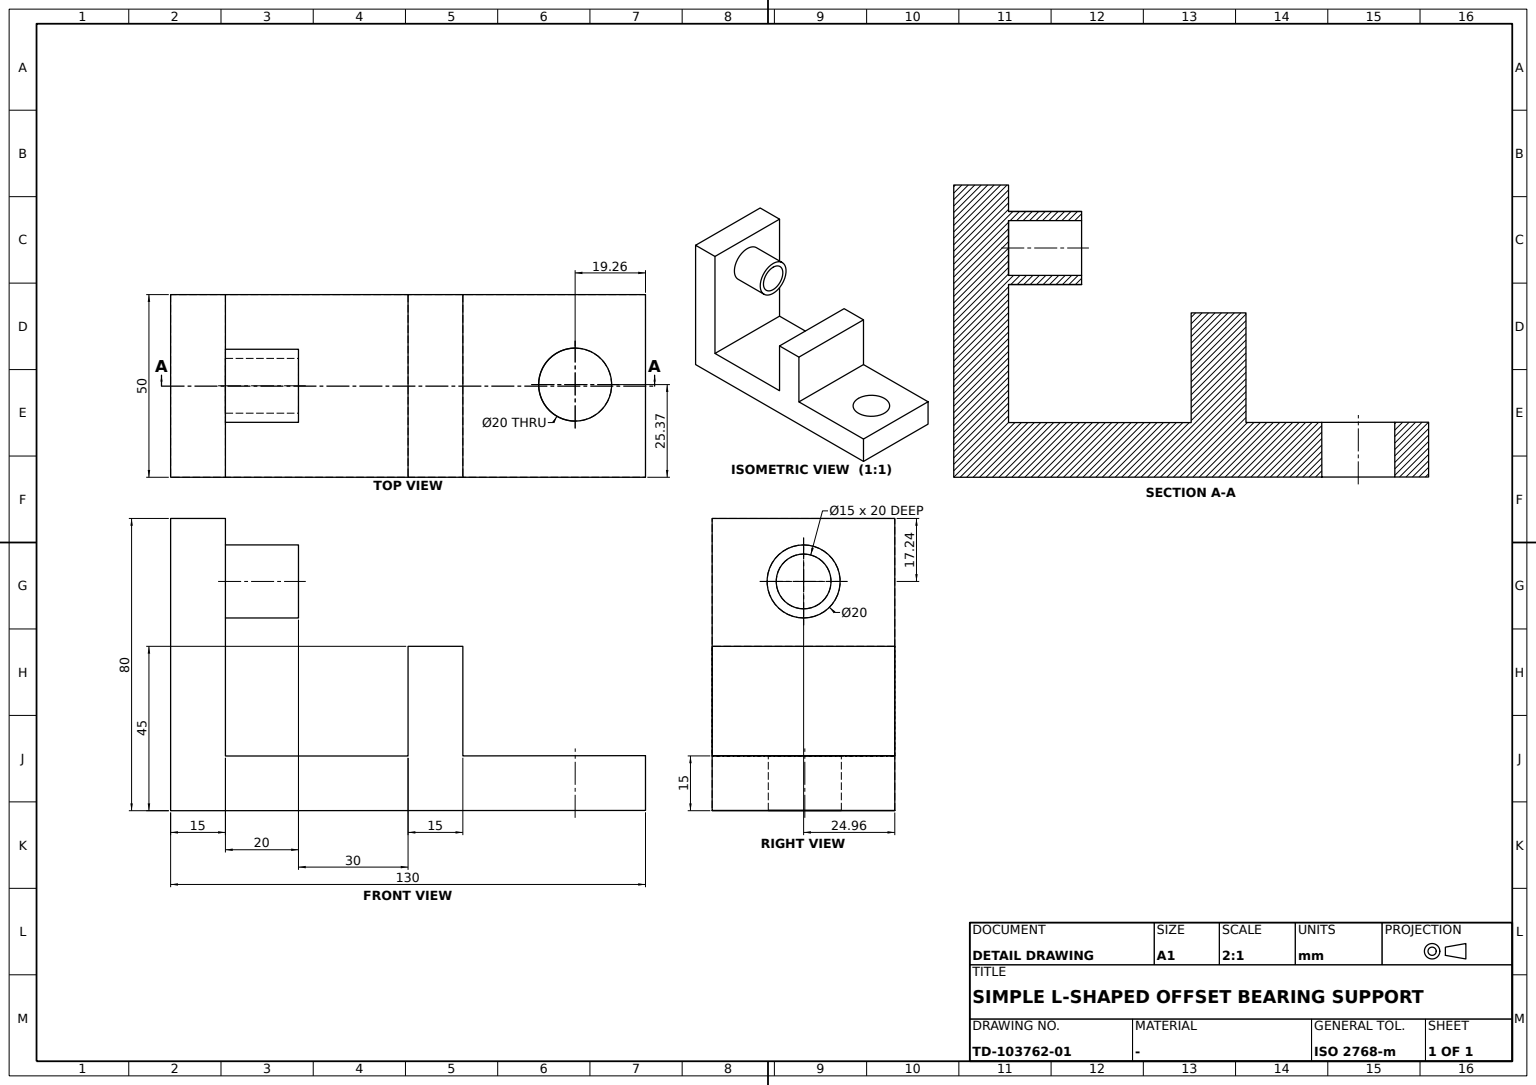
CATIA V5 part; units mm, degrees
sketch "Sketch1" plane through (0, 0, 0) normal (1, 0, 0) x (0, 1, 0)
  line L0 (0, 0) -> (130, 0.0732)
  line L1 (130, 0.0732) -> (130, 15.0732)
  line L2 (130, 15.0732) -> (80, 14.9978)
  line L3 (80, 14.9978) -> (80, 44.9978)
  line L4 (80, 44.9978) -> (65, 44.9978)
  line L5 (65, 44.9978) -> (65, 14.9751)
  line L6 (0, 0) -> (0, 80)
  line L7 (0, 80) -> (15, 80)
  line L8 (15, 80) -> (15, 14.9751)
  line L9 (65, 14.9751) -> (15, 14.9751)
  dimension "length L0" = 130
  dimension "length L1" = 15
  dimension "length L2" = 50
  dimension "length L3" = 30
  dimension "length L4" = 15
  dimension "length L6" = 80
  dimension "length L7" = 15
extrude "Pad1" add sketch "Sketch1" along normal blind 50
sketch "Sketch3" plane through (0, 15, 0) normal (0, 1, 0) x (-1, 0, 0)
  circle A0 centre (-24.9594, 62.7568) radius 10
  circle A1 centre (-24.9594, 62.7568) radius 7.5
  dimension "radius A0" = 10
  dimension "radius A1" = 7.5
extrude "Pad2" add sketch "Sketch3" along normal blind 20
sketch "Sketch4" plane through (0, -0.0225, 14.8771) normal (0, -0.0015, 1) x (1, 0, 0)
  circle A0 centre (24.6324, 110.7606) radius 10
  dimension "radius A0" = 10
extrude "Pocket1" cut sketch "Sketch4" against normal blind 20
sketch "Sketch2" plane through (0, -0.0225, 14.877) normal (0, -0.0015, 1) x (1, 0, 0)
  point P0 (50, 129.9245)
  line L0 (25, 129.9747) -> (25, 129.9245)
  point P1 (25, 104.9747)
